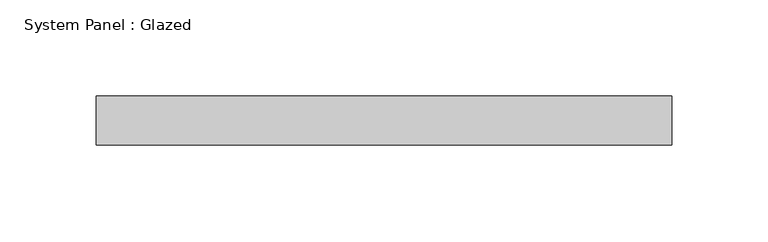
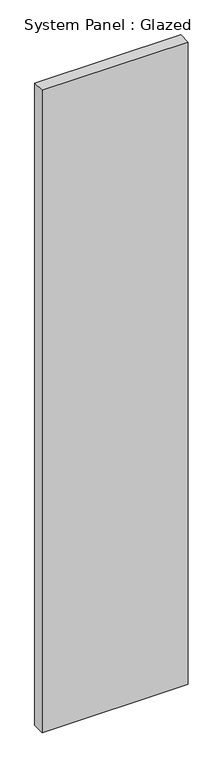
"""IFC4 building model written with IfcOpenShell, lengths in millimetres: plate geometry, System Panel : Glazed."""

from ifc_helpers import new_model, si_unit, origin, origin_with_axes, place, context, project, spatial, polyline, outline, extrude, source, transform, mapped, element, save


def system_panel_glazed_8a1f71ef(model_context):
    return source(origin(), model_context, "Body", "SweptSolid", [
        extrude(outline(polyline([(149.225, 19.05), (-149.225, 19.05), (-149.225, 44.45), (149.225, 44.45), (149.225, 19.05)])), origin_with_axes(), (0.0, 0.0, 1.0), 1385.8617517),
    ])


if __name__ == "__main__":
    model = new_model("IFC4")
    model_context = context("Model", 3, world=origin())
    ifc_project = project(units=[si_unit("LENGTHUNIT", "METRE", prefix="MILLI")], contexts=[model_context])
    site = spatial("IfcSite", under=ifc_project)
    building = spatial("IfcBuilding", under=site)
    placement = place(None, origin())
    system_panel_glazed_shape = system_panel_glazed_8a1f71ef(model_context)
    element("IfcPlate", 1, ObjectType="System Panel : Glazed", at=placement, inside=building, context=model_context, shape_type="MappedRepresentation", body=[
        mapped(system_panel_glazed_shape, transform((0.0, 0.0, 0.0), x_axis=(1.0, 0.0, 0.0), y_axis=(0.0, 1.0, 0.0), z_axis=(0.0, 0.0, 1.0))),
    ])
    save(model, "model.ifc")

# Revit data of these elements
# Type "System Panel : Glazed"
#   Construction Type Id = "GSP4R"
#   Analytic Construction = "1/8 in Pilkington single glazing"
#   Visual Light Transmittance = 0.9
#   Solar Heat Gain Coefficient = 0.86
#   Heat Transfer Coefficient (U) = 1.18115 BTU/(h·ft²·°F)
#   Define Thermal Properties by = 1
# Element 1 (IfcPlate, "System Panel : Glazed")
#   Materials on its faces: "Glass"
# Materials
#   "Glass": class "Glass", colour RGB 0 128 192, transparency 0.75, Description = "Soda Lime Glass", Cost = 0
